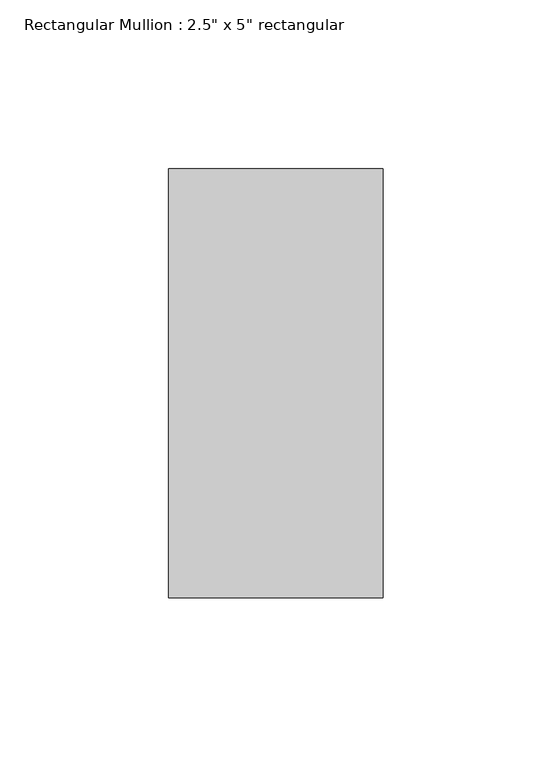
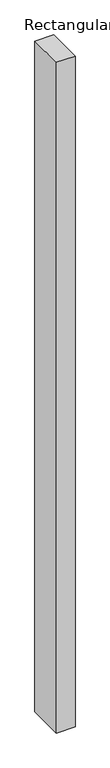
"""IFC4 building model written with IfcOpenShell, lengths in millimetres: member geometry."""

from ifc_helpers import new_model, si_unit, frame, origin, place, context, project, spatial, polyline, outline, extrude, source, transform, mapped, element, save


def member_360d9ee7(model_context):
    return source(origin(), model_context, "Body", "SweptSolid", [
        extrude(outline(polyline([(0.0, 63.5), (0.0, -63.5), (-63.5, -63.5), (-63.5, 63.5), (0.0, 63.5)])), frame((0.0, 0.0, -2417.9442596), z_axis=(0.0, 0.0, 1.0), x_axis=(1.0, 0.0, 0.0)), (0.0, 0.0, 1.0), 2417.9442596),
    ])


if __name__ == "__main__":
    model = new_model("IFC4")
    model_context = context("Model", 3, world=origin())
    ifc_project = project(units=[si_unit("LENGTHUNIT", "METRE", prefix="MILLI")], contexts=[model_context])
    site = spatial("IfcSite", under=ifc_project)
    building = spatial("IfcBuilding", under=site)
    placement = place(None, origin())
    member_shape = member_360d9ee7(model_context)
    element("IfcMember", 1, ObjectType="Rectangular Mullion : 2.5\" x 5\" rectangular", at=placement, inside=building, context=model_context, shape_type="MappedRepresentation", body=[
        mapped(member_shape, transform((0.0, 0.0, 0.0), x_axis=(1.0, 0.0, 0.0), y_axis=(0.0, 1.0, 0.0), z_axis=(0.0, 0.0, 1.0))),
    ])
    save(model, "model.ifc")

# Revit data of these elements
# Type "Rectangular Mullion : 2.5\" x 5\" rectangular"
#   built-in parameter 1007304 = 0.416667 (stored number, unit not read)
#   built-in parameter 1007301 = 0.104167 (stored number, unit not read)
#   built-in parameter 1007300 = 0.104167 (stored number, unit not read)
# Element 1 (IfcMember, "Rectangular Mullion : 2.5\" x 5\" rectangular")
#   Materials on its faces: "Aluminum"
# Materials
#   "Aluminum": class "Metal", colour RGB 247 247 247, transparency 0, Description = "Aluminum 6061", Cost = 0
